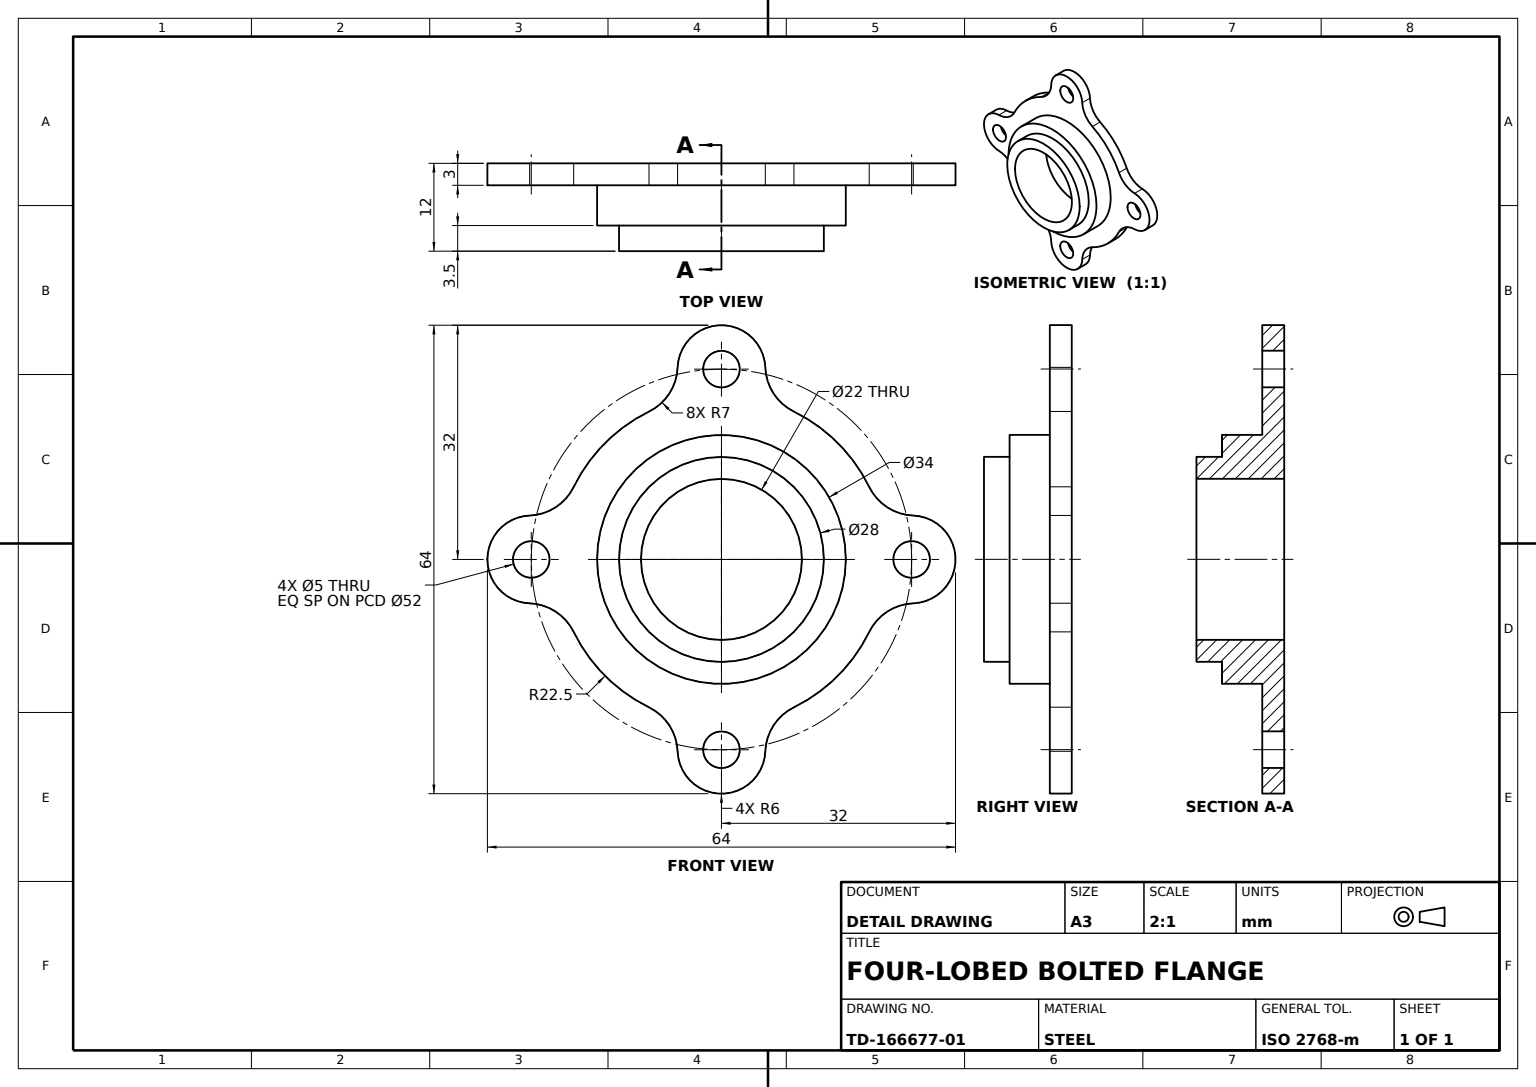
from build123d import *

# Parameters (mm, degrees)
LUG_FLANGE_DEPTH            = 3
HUB_SKETCH_R                = 17
HUB_BOSS_DEPTH              = 5.5
SPIGOT_SKETCH_R             = 14
LOCATING_SPIGOT_DEPTH       = 3.5
BEARING_BORE_SKETCH_R       = 11
BEARING_BORE_DEPTH          = 15
LUG_HOLES_SKETCH_R          = 2.5
LUG_MOUNTING_HOLES_4X_DEPTH = 15


with BuildPart() as part:
    # Flange Profile Sketch → Lug Flange (new body)
    with BuildSketch(Plane.XY):
        with BuildLine():
            ThreePointArc((9.908335055, -20.200863755), (15.909902577, -15.909902577), (20.200863755, -9.908335055))
            ThreePointArc((20.200863755, -9.908335055), (22.672432853, -7.120669901), (26.224112426, -5.995813007))
            ThreePointArc((26.224112426, -5.995813007), (32, 0), (26.224112426, 5.995813007))
            ThreePointArc((26.224112426, 5.995813007), (22.672432853, 7.120669901), (20.200863755, 9.908335055))
            ThreePointArc((20.200863755, 9.908335055), (15.909902577, 15.909902577), (9.908335055, 20.200863755))
            ThreePointArc((9.908335055, 20.200863755), (7.120669901, 22.672432853), (5.995813007, 26.224112426))
            ThreePointArc((5.995813007, 26.224112426), (0, 32), (-5.995813007, 26.224112426))
            ThreePointArc((-5.995813007, 26.224112426), (-7.120669901, 22.672432853), (-9.908335055, 20.200863755))
            ThreePointArc((-9.908335055, 20.200863755), (-15.909902577, 15.909902577), (-20.200863755, 9.908335055))
            ThreePointArc((-20.200863755, 9.908335055), (-22.672432853, 7.120669901), (-26.224112426, 5.995813007))
            ThreePointArc((-26.224112426, 5.995813007), (-32, 0), (-26.224112426, -5.995813007))
            ThreePointArc((-26.224112426, -5.995813007), (-22.672432853, -7.120669901), (-20.200863755, -9.908335055))
            ThreePointArc((-20.200863755, -9.908335055), (-15.909902577, -15.909902577), (-9.908335055, -20.200863755))
            ThreePointArc((-9.908335055, -20.200863755), (-7.120669901, -22.672432853), (-5.995813007, -26.224112426))
            ThreePointArc((-5.995813007, -26.224112426), (0, -32), (5.995813007, -26.224112426))
            ThreePointArc((5.995813007, -26.224112426), (7.120669901, -22.672432853), (9.908335055, -20.200863755))
        make_face()
    extrude(amount=LUG_FLANGE_DEPTH)

    # Hub Sketch → Hub Boss (add)
    with BuildSketch(Plane.XY.offset(3)):
        with Locations(Location((0, 0, 0), (0, 0, 180))):
            Circle(HUB_SKETCH_R)
    extrude(amount=HUB_BOSS_DEPTH)

    # Spigot Sketch → Locating Spigot (add)
    with BuildSketch(Plane.XY.offset(8.5)):
        Circle(SPIGOT_SKETCH_R)
    extrude(amount=LOCATING_SPIGOT_DEPTH)

    # Bearing Bore Sketch → Bearing Bore (cut)
    with BuildSketch(Plane.XY.offset(12)):
        Circle(BEARING_BORE_SKETCH_R)
    extrude(amount=-BEARING_BORE_DEPTH, mode=Mode.SUBTRACT)

    # Lug Holes Sketch → Lug Mounting Holes 4x (cut)
    with BuildSketch(Plane.XY.offset(3)):
        with Locations((-26, 0)):
            Circle(LUG_HOLES_SKETCH_R)
        with Locations((0, 26)):
            Circle(LUG_HOLES_SKETCH_R)
        with Locations((26, 0)):
            Circle(LUG_HOLES_SKETCH_R)
        with Locations((0, -26)):
            Circle(LUG_HOLES_SKETCH_R)
    extrude(amount=-LUG_MOUNTING_HOLES_4X_DEPTH, mode=Mode.SUBTRACT)


solid = part.part
